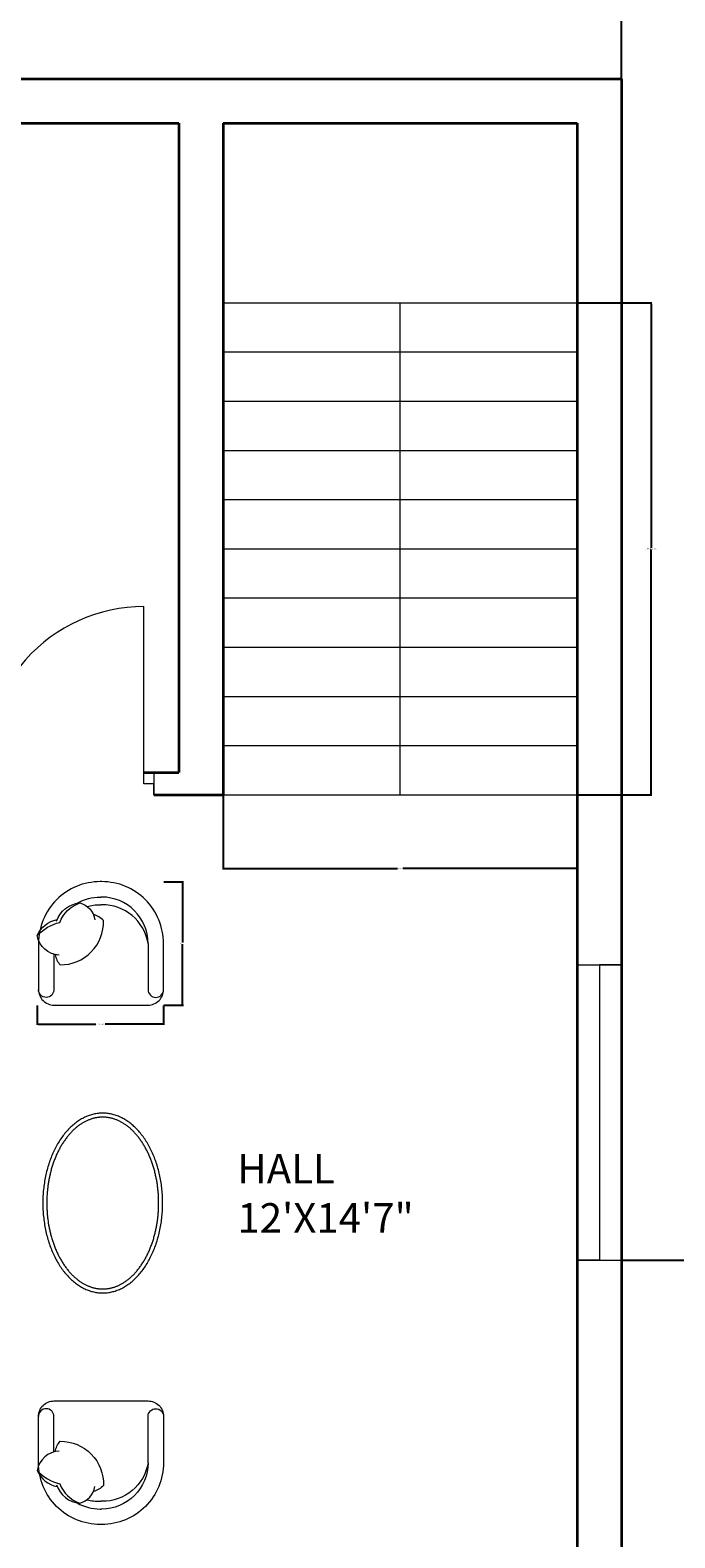
# Model space of a CAD drawing. Units: inches. Extents: x 2003 to 3241, y 1726 to 2849.
# Tile 3 of 7: x 2186 to 2317, y 2073 to 2380. Entities that reach past the tile are written whole.
import ezdxf

# ---------------------------------------------------------------- set-up
doc = ezdxf.new("R2010")
doc.units = ezdxf.units.IN
for name, color, linetype, lineweight in [('A-ANNO-DIMS', 2, 'Continuous', 18), ('A-AREA-IDEN', 7, 'Continuous', 18), ('A-DOOR', 3, 'Continuous', 18), ('A-FLOR-STRS', 7, 'Continuous', 18), ('A-FURN', 8, 'Continuous', 13), ('A-GLAZ', 4, 'Continuous', 18), ('A-WALL', 7, 'Continuous', 35)]:
    doc.layers.add(name, color=color, linetype=linetype, lineweight=lineweight)
doc.styles.get("Standard").update_dxf_attribs({"font": 'arial.ttf'})
doc.dimstyles.get("Standard").update_dxf_attribs({"dimtxt": 0.18, "dimasz": 0.18, "dimexe": 0.18, "dimexo": 0.0625, "dimgap": 0.09, "dimtad": 0, "dimtih": 1, "dimtoh": 1, "dimdec": 4, "dimzin": 0, "dimdsep": 46, "dimtxsty": 'Standard', "dimcen": 0.09, "dimadec": 0, "dimazin": 0, "dimtfac": 1, "dimtdec": 4, "dimtofl": 0, "dimtmove": 0, "dimatfit": 3, "dimfxl": 1, "dimtolj": 1, "dimtzin": 0, "dimarcsym": 0})

# ---------------------------------------------------------------- blocks, each defined once
blk = doc.blocks.new('WIN-60-HALL')
for p, q in [((0, 60), (9, 60)), ((9, 60), (4.5, 60)), ((4.5, 60), (4.5, 0)), ((4.5, 0), (0, 0)), ((0, 0), (9, 0)), ((9, 0), (9, 0))]:
    blk.add_line(p, q)
blk = doc.blocks.new('DOOR-BEDROOM')
for p, q in [((34.02, 2.25), (34.02, 38.25)), ((0, 4.5), (0, 0)), ((36.02, 4.5), (36.02, 0)), ((0, 0), (0, 2.25)), ((0, 2.25), (2, 2.25)), ((36.02, 2.25), (34.02, 2.25)), ((36.02, 0), (36.02, 2.25))]:
    blk.add_line(p, q)
blk.add_arc((34.02, 6.01), 32.24, 90, 186.689)
blk = doc.blocks.new('STAIR-GROUND-RUN')
for p, q in [((0, 100), (72, 100)), ((36, 97.06), (36, 100)), ((36, 0), (36, 97.06)), ((0, 90), (72, 90)), ((0, 80), (72, 80)), ((0, 70), (72, 70)), ((0, 60), (72, 60)), ((0, 50), (72, 50)), ((0, 40), (72, 40)), ((0, 30), (72, 30)), ((0, 20), (72, 20)), ((0, 10), (72, 10)), ((0, 0), (72, 0))]:
    blk.add_line(p, q)
blk = doc.blocks.new('CHAIR-LOUNGE')
at = {"ltscale": 0.03}
blk.add_lwpolyline([(12.96, 0), (22.53, 0, 0.414214), (25.67, 3.14), (25.67, 12.55, 0.414214), (13.12, 25.1), (12.96, 25.1), (12.81, 25.1, 0.414214), (0.26, 12.55), (0.26, 3.14, 0.414214), (3.39, 0), (12.96, 0)], format="xyb", dxfattribs=at)
for points in [[(8.13, 20.72, -0.130591), (12.81, 21.96), (12.96, 21.96)], [(22.53, 12.55, 0.414214), (13.12, 21.96), (12.96, 21.96)], [(0, 14.13, -0.14773), (4.58, 16.83, -0.213343), (8.63, 20.78, -0.178662)], [(3.7, 10.28, 0.165541), (4.67, 8.2, 0.425989), (13.48, 17.19, 0.121523), (11.39, 18.43, -7.115464)], [(3.95, 17.04, -0.306663), (8.63, 20.78, -0.30633), (11.69, 17.37, 0.872847)], [(10.13, 20.06, -0.072384), (12.81, 20.39), (12.96, 20.39)], [(22.53, 12.55, 0.372719), (13.12, 20.39), (12.96, 20.39)], [(4.49, 10.18, -0.356772), (0, 14.13, -0.249542), (4.07, 17.39, 9.61688)], [(22.53, 12.55), (22.53, 3.14, 0.414214), (24.1, 1.57), (24.1, 1.57, 0.414214), (25.67, 3.14)], [(3.39, 10.35), (3.39, 3.14, -0.414214), (1.83, 1.57), (1.83, 1.57, -0.414214), (0.26, 3.14)]]:
    blk.add_lwpolyline(points, format="xyb")
blk = doc.blocks.new('*D52')
at = {"layer": 'A-ANNO-DIMS', "color": 0, "lineweight": -2, "transparency": 16777216}
for p, q in [((2296.84, 2324.41), (2311.96, 2324.41)), ((2311.78, 2324.23), (2311.78, 2274.6)), ((2311.78, 2224.59), (2311.78, 2274.23)), ((2296.84, 2224.41), (2311.96, 2224.41))]:
    blk.add_line(p, q, dxfattribs=at)
at = {"layer": 'A-ANNO-DIMS', "color": 0, "transparency": 16777216}
for points in [[(2311.75, 2324.23), (2311.81, 2324.23), (2311.78, 2324.41)], [(2311.75, 2224.59), (2311.81, 2224.59), (2311.78, 2224.41)]]:
    blk.add_solid(points, dxfattribs=at)
at = {"layer": 'Defpoints', "color": 0, "transparency": 16777216}
for p in [(2296.78, 2324.41), (2311.78, 2324.41), (2296.78, 2224.41)]:
    blk.add_point(p, dxfattribs=at)
at = {"layer": 'A-ANNO-DIMS', "color": 0, "transparency": 16777216, "insert": (2311.78, 2274.41), "char_height": 0.18, "attachment_point": 5}
blk.add_mtext('\\A1;STAIR RUN 100 TYP.', dxfattribs=at)
blk = doc.blocks.new('*D53')
at = {"layer": 'A-ANNO-DIMS', "color": 0, "lineweight": -2, "transparency": 16777216}
for p, q in [((2224.78, 2224.35), (2224.78, 2209.23)), ((2296.78, 2224.35), (2296.78, 2209.23)), ((2224.96, 2209.41), (2260.25, 2209.41)), ((2296.6, 2209.41), (2261.31, 2209.41))]:
    blk.add_line(p, q, dxfattribs=at)
at = {"layer": 'A-ANNO-DIMS', "color": 0, "transparency": 16777216}
for points in [[(2224.96, 2209.44), (2224.96, 2209.38), (2224.78, 2209.41)], [(2296.6, 2209.44), (2296.6, 2209.38), (2296.78, 2209.41)]]:
    blk.add_solid(points, dxfattribs=at)
at = {"layer": 'Defpoints', "color": 0, "transparency": 16777216}
for p in [(2224.78, 2224.41), (2296.78, 2224.41), (2296.78, 2209.41)]:
    blk.add_point(p, dxfattribs=at)
at = {"layer": 'A-ANNO-DIMS', "color": 0, "transparency": 16777216, "insert": (2260.78, 2209.41), "char_height": 0.18, "attachment_point": 5}
blk.add_mtext('\\A1;72 TYP.', dxfattribs=at)
blk = doc.blocks.new('*D62')
at = {"layer": 'A-ANNO-DIMS', "color": 0, "lineweight": -2, "transparency": 16777216}
for p, q in [((2187.02, 2181.59), (2187.02, 2177.62)), ((2212.69, 2181.59), (2212.69, 2177.62)), ((2187.2, 2177.8), (2198.9, 2177.8)), ((2212.51, 2177.8), (2200.81, 2177.8))]:
    blk.add_line(p, q, dxfattribs=at)
at = {"layer": 'A-ANNO-DIMS', "color": 0, "transparency": 16777216}
for points in [[(2187.2, 2177.83), (2187.2, 2177.77), (2187.02, 2177.8)], [(2212.51, 2177.83), (2212.51, 2177.77), (2212.69, 2177.8)]]:
    blk.add_solid(points, dxfattribs=at)
at = {"layer": 'Defpoints', "color": 0, "transparency": 16777216}
for p in [(2187.02, 2181.65), (2212.69, 2181.65), (2212.69, 2177.8)]:
    blk.add_point(p, dxfattribs=at)
at = {"layer": 'A-ANNO-DIMS', "color": 0, "transparency": 16777216, "insert": (2199.85, 2177.8), "char_height": 0.18, "attachment_point": 5}
blk.add_mtext('\\A1;CHAIR 26 TYP.', dxfattribs=at)
blk = doc.blocks.new('*D63')
at = {"layer": 'A-ANNO-DIMS', "color": 0, "lineweight": -2, "transparency": 16777216}
for p, q in [((2212.75, 2206.75), (2216.72, 2206.75)), ((2216.54, 2206.57), (2216.54, 2194.38)), ((2216.54, 2181.83), (2216.54, 2194.02)), ((2212.75, 2181.65), (2216.72, 2181.65))]:
    blk.add_line(p, q, dxfattribs=at)
at = {"layer": 'A-ANNO-DIMS', "color": 0, "transparency": 16777216}
for points in [[(2216.51, 2206.57), (2216.57, 2206.57), (2216.54, 2206.75)], [(2216.51, 2181.83), (2216.57, 2181.83), (2216.54, 2181.65)]]:
    blk.add_solid(points, dxfattribs=at)
at = {"layer": 'Defpoints', "color": 0, "transparency": 16777216}
for p in [(2212.69, 2206.75), (2216.54, 2206.75), (2212.69, 2181.65)]:
    blk.add_point(p, dxfattribs=at)
at = {"layer": 'A-ANNO-DIMS', "color": 0, "transparency": 16777216, "insert": (2216.54, 2194.2), "char_height": 0.18, "attachment_point": 5}
blk.add_mtext('\\A1;25 TYP.', dxfattribs=at)
blk = doc.blocks.new('*D64')
at = {"layer": 'A-ANNO-DIMS', "color": 0, "lineweight": -2, "transparency": 16777216}
for p, q in [((2089.78, 2369.98), (2089.78, 2399.74)), ((2089.96, 2399.56), (2197.49, 2399.56)), ((2305.6, 2399.56), (2198.07, 2399.56)), ((2305.78, 2369.98), (2305.78, 2399.74))]:
    blk.add_line(p, q, dxfattribs=at)
at = {"layer": 'A-ANNO-DIMS', "color": 0, "transparency": 16777216}
for points in [[(2089.96, 2399.59), (2089.96, 2399.53), (2089.78, 2399.56)], [(2305.6, 2399.59), (2305.6, 2399.53), (2305.78, 2399.56)]]:
    blk.add_solid(points, dxfattribs=at)
at = {"layer": 'Defpoints', "color": 0, "transparency": 16777216}
for p in [(2305.78, 2399.56), (2089.78, 2369.91), (2305.78, 2369.91)]:
    blk.add_point(p, dxfattribs=at)
at = {"layer": 'A-ANNO-DIMS', "color": 0, "transparency": 16777216, "insert": (2197.78, 2399.56), "char_height": 0.18, "attachment_point": 5}
blk.add_mtext('\\A1;216', dxfattribs=at)
blk = doc.blocks.new('*D67')
at = {"layer": 'A-ANNO-DIMS', "color": 0, "lineweight": -2, "transparency": 16777216}
for p, q in [((2305.84, 2129.81), (2335.61, 2129.81)), ((2335.43, 2129.63), (2335.43, 2026.55)), ((2335.43, 1923.09), (2335.43, 2026.18)), ((2305.84, 1922.91), (2335.61, 1922.91))]:
    blk.add_line(p, q, dxfattribs=at)
at = {"layer": 'A-ANNO-DIMS', "color": 0, "transparency": 16777216}
for points in [[(2335.4, 2129.63), (2335.46, 2129.63), (2335.43, 2129.81)], [(2335.4, 1923.09), (2335.46, 1923.09), (2335.43, 1922.91)]]:
    blk.add_solid(points, dxfattribs=at)
at = {"layer": 'Defpoints', "color": 0, "transparency": 16777216}
for p in [(2305.78, 2129.81), (2335.43, 2129.81), (2305.78, 1922.91)]:
    blk.add_point(p, dxfattribs=at)
at = {"layer": 'A-ANNO-DIMS', "color": 0, "transparency": 16777216, "insert": (2335.43, 2026.36), "char_height": 0.18, "attachment_point": 5}
blk.add_mtext('\\A1;206.9', dxfattribs=at)

msp = doc.modelspace()

# ---------------------------------------------------------------- linework, layer by layer
at = {"layer": 'A-FURN', "ltscale": 0.03}
msp.add_polyline3d([(2200.3301, 2159.6931, 0), (2200.0996, 2159.6898, 0), (2199.8692, 2159.68, 0), (2199.639, 2159.6637, 0), (2199.409, 2159.6408, 0), (2199.1794, 2159.6114, 0), (2198.9501, 2159.5755, 0), (2198.7214, 2159.533, 0), (2198.4932, 2159.4841, 0), (2198.2657, 2159.4287, 0), (2198.0389, 2159.3669, 0), (2197.813, 2159.2987, 0), (2197.5879, 2159.224, 0), (2197.3638, 2159.143, 0), (2197.1408, 2159.0556, 0), (2196.919, 2158.9619, 0), (2196.6983, 2158.862, 0), (2196.479, 2158.7557, 0), (2196.261, 2158.6433, 0), (2196.0445, 2158.5247, 0), (2195.8296, 2158.4, 0), (2195.6162, 2158.2692, 0), (2195.4045, 2158.1324, 0), (2195.1946, 2157.9896, 0), (2194.9866, 2157.8409, 0), (2194.7804, 2157.6862, 0), (2194.5762, 2157.5258, 0), (2194.3741, 2157.3596, 0), (2194.1742, 2157.1876, 0), (2193.9764, 2157.0101, 0), (2193.7809, 2156.8269, 0), (2193.5878, 2156.6383, 0), (2193.397, 2156.4442, 0), (2193.2088, 2156.2447, 0), (2193.0231, 2156.0399, 0), (2192.84, 2155.8298, 0), (2192.6596, 2155.6146, 0), (2192.482, 2155.3944, 0), (2192.3071, 2155.1691, 0), (2192.1352, 2154.9389, 0), (2191.9661, 2154.7038, 0), (2191.8001, 2154.464, 0), (2191.6371, 2154.2196, 0), (2191.4773, 2153.9705, 0), (2191.3206, 2153.717, 0), (2191.1671, 2153.459, 0), (2191.0169, 2153.1968, 0), (2190.87, 2152.9303, 0), (2190.7266, 2152.6597, 0), (2190.5866, 2152.3851, 0), (2190.45, 2152.1065, 0), (2190.317, 2151.8242, 0), (2190.1876, 2151.5381, 0), (2190.0618, 2151.2483, 0), (2189.9397, 2150.9551, 0), (2189.8214, 2150.6585, 0), (2189.7068, 2150.3585, 0), (2189.5959, 2150.0553, 0), (2189.489, 2149.7491, 0), (2189.3859, 2149.4399, 0), (2189.2867, 2149.1278, 0), (2189.1915, 2148.8129, 0), (2189.1003, 2148.4954, 0), (2189.0131, 2148.1754, 0), (2188.93, 2147.8529, 0), (2188.8509, 2147.5282, 0), (2188.776, 2147.2012, 0), (2188.7052, 2146.8722, 0), (2188.6385, 2146.5412, 0), (2188.5761, 2146.2084, 0), (2188.5178, 2145.8739, 0), (2188.4638, 2145.5378, 0), (2188.414, 2145.2002, 0), (2188.3685, 2144.8613, 0), (2188.3273, 2144.5212, 0), (2188.2904, 2144.1799, 0), (2188.2578, 2143.8376, 0), (2188.2295, 2143.4945, 0), (2188.2055, 2143.1507, 0), (2188.1859, 2142.8062, 0), (2188.1707, 2142.4612, 0), (2188.1598, 2142.1159, 0), (2188.1532, 2141.7703, 0), (2188.1511, 2141.4246, 0), (2188.1532, 2141.0788, 0), (2188.1598, 2140.7332, 0), (2188.1707, 2140.3879, 0), (2188.1859, 2140.0429, 0), (2188.2055, 2139.6984, 0), (2188.2295, 2139.3546, 0), (2188.2578, 2139.0115, 0), (2188.2904, 2138.6692, 0), (2188.3273, 2138.3279, 0), (2188.3685, 2137.9878, 0), (2188.414, 2137.6489, 0), (2188.4638, 2137.3113, 0), (2188.5178, 2136.9752, 0), (2188.5761, 2136.6407, 0), (2188.6385, 2136.3079, 0), (2188.7052, 2135.9769, 0), (2188.776, 2135.6479, 0), (2188.8509, 2135.3209, 0), (2188.93, 2134.9962, 0), (2189.0131, 2134.6737, 0), (2189.1003, 2134.3537, 0), (2189.1915, 2134.0362, 0), (2189.2867, 2133.7213, 0), (2189.3859, 2133.4092, 0), (2189.489, 2133.1, 0), (2189.5959, 2132.7938, 0), (2189.7068, 2132.4906, 0), (2189.8214, 2132.1906, 0), (2189.9397, 2131.894, 0), (2190.0618, 2131.6008, 0), (2190.1876, 2131.311, 0), (2190.317, 2131.025, 0), (2190.45, 2130.7426, 0), (2190.5866, 2130.464, 0), (2190.7266, 2130.1894, 0), (2190.87, 2129.9188, 0), (2191.0169, 2129.6523, 0), (2191.1671, 2129.3901, 0), (2191.3206, 2129.1321, 0), (2191.4773, 2128.8786, 0), (2191.6371, 2128.6295, 0), (2191.8001, 2128.3851, 0), (2191.9661, 2128.1453, 0), (2192.1352, 2127.9102, 0), (2192.3071, 2127.68, 0), (2192.482, 2127.4547, 0), (2192.6596, 2127.2345, 0), (2192.84, 2127.0193, 0), (2193.0231, 2126.8092, 0), (2193.2088, 2126.6044, 0), (2193.397, 2126.4049, 0), (2193.5878, 2126.2108, 0), (2193.7809, 2126.0222, 0), (2193.9764, 2125.839, 0), (2194.1742, 2125.6615, 0), (2194.3741, 2125.4895, 0), (2194.5762, 2125.3233, 0), (2194.7804, 2125.1629, 0), (2194.9866, 2125.0082, 0), (2195.1946, 2124.8595, 0), (2195.4045, 2124.7167, 0), (2195.6162, 2124.5799, 0), (2195.8296, 2124.4491, 0), (2196.0445, 2124.3244, 0), (2196.261, 2124.2058, 0), (2196.479, 2124.0934, 0), (2196.6983, 2123.9871, 0), (2196.919, 2123.8872, 0), (2197.1408, 2123.7935, 0), (2197.3638, 2123.7061, 0), (2197.5879, 2123.6251, 0), (2197.813, 2123.5504, 0), (2198.0389, 2123.4822, 0), (2198.2657, 2123.4204, 0), (2198.4932, 2123.365, 0), (2198.7214, 2123.3161, 0), (2198.9501, 2123.2736, 0), (2199.1794, 2123.2377, 0), (2199.409, 2123.2083, 0), (2199.639, 2123.1854, 0), (2199.8692, 2123.1691, 0), (2200.0996, 2123.1593, 0), (2200.3301, 2123.156, 0), (2200.5606, 2123.1593, 0), (2200.791, 2123.1691, 0), (2201.0212, 2123.1854, 0), (2201.2512, 2123.2083, 0), (2201.4808, 2123.2377, 0), (2201.7101, 2123.2736, 0), (2201.9388, 2123.3161, 0), (2202.167, 2123.365, 0), (2202.3945, 2123.4204, 0), (2202.6213, 2123.4822, 0), (2202.8472, 2123.5504, 0), (2203.0723, 2123.6251, 0), (2203.2964, 2123.7061, 0), (2203.5194, 2123.7935, 0), (2203.7412, 2123.8872, 0), (2203.9619, 2123.9871, 0), (2204.1812, 2124.0934, 0), (2204.3992, 2124.2058, 0), (2204.6157, 2124.3244, 0), (2204.8306, 2124.4491, 0), (2205.044, 2124.5799, 0), (2205.2557, 2124.7167, 0), (2205.4656, 2124.8595, 0), (2205.6736, 2125.0082, 0), (2205.8798, 2125.1629, 0), (2206.084, 2125.3233, 0), (2206.2861, 2125.4895, 0), (2206.486, 2125.6615, 0), (2206.6838, 2125.839, 0), (2206.8793, 2126.0222, 0), (2207.0724, 2126.2108, 0), (2207.2632, 2126.4049, 0), (2207.4514, 2126.6044, 0), (2207.6371, 2126.8092, 0), (2207.8202, 2127.0193, 0), (2208.0006, 2127.2345, 0), (2208.1782, 2127.4547, 0), (2208.3531, 2127.68, 0), (2208.525, 2127.9102, 0), (2208.6941, 2128.1453, 0), (2208.8601, 2128.3851, 0), (2209.0231, 2128.6295, 0), (2209.183, 2128.8786, 0), (2209.3396, 2129.1321, 0), (2209.4931, 2129.3901, 0), (2209.6433, 2129.6523, 0), (2209.7902, 2129.9188, 0), (2209.9336, 2130.1894, 0), (2210.0736, 2130.464, 0), (2210.2102, 2130.7426, 0), (2210.3432, 2131.025, 0), (2210.4726, 2131.311, 0), (2210.5984, 2131.6008, 0), (2210.7205, 2131.894, 0), (2210.8388, 2132.1906, 0), (2210.9534, 2132.4906, 0), (2211.0643, 2132.7938, 0), (2211.1712, 2133.1, 0), (2211.2743, 2133.4092, 0), (2211.3735, 2133.7213, 0), (2211.4687, 2134.0362, 0), (2211.5599, 2134.3537, 0), (2211.6471, 2134.6737, 0), (2211.7302, 2134.9962, 0), (2211.8093, 2135.3209, 0), (2211.8842, 2135.6479, 0), (2211.955, 2135.9769, 0), (2212.0217, 2136.3079, 0), (2212.0841, 2136.6407, 0), (2212.1424, 2136.9752, 0), (2212.1964, 2137.3113, 0), (2212.2462, 2137.6489, 0), (2212.2917, 2137.9878, 0), (2212.3329, 2138.3279, 0), (2212.3698, 2138.6692, 0), (2212.4024, 2139.0115, 0), (2212.4307, 2139.3546, 0), (2212.4547, 2139.6984, 0), (2212.4743, 2140.0429, 0), (2212.4895, 2140.3879, 0), (2212.5004, 2140.7332, 0), (2212.507, 2141.0788, 0), (2212.5091, 2141.4246, 0), (2212.507, 2141.7703, 0), (2212.5004, 2142.1159, 0), (2212.4895, 2142.4612, 0), (2212.4743, 2142.8062, 0), (2212.4547, 2143.1507, 0), (2212.4307, 2143.4945, 0), (2212.4024, 2143.8376, 0), (2212.3698, 2144.1799, 0), (2212.3329, 2144.5212, 0), (2212.2917, 2144.8613, 0), (2212.2462, 2145.2002, 0), (2212.1964, 2145.5378, 0), (2212.1424, 2145.8739, 0), (2212.0841, 2146.2084, 0), (2212.0217, 2146.5412, 0), (2211.955, 2146.8722, 0), (2211.8842, 2147.2012, 0), (2211.8093, 2147.5282, 0), (2211.7302, 2147.8529, 0), (2211.6471, 2148.1754, 0), (2211.5599, 2148.4954, 0), (2211.4687, 2148.8129, 0), (2211.3735, 2149.1278, 0), (2211.2743, 2149.4399, 0), (2211.1712, 2149.7491, 0), (2211.0643, 2150.0553, 0), (2210.9534, 2150.3585, 0), (2210.8388, 2150.6585, 0), (2210.7205, 2150.9551, 0), (2210.5984, 2151.2483, 0), (2210.4726, 2151.5381, 0), (2210.3432, 2151.8242, 0), (2210.2102, 2152.1065, 0), (2210.0736, 2152.3851, 0), (2209.9336, 2152.6597, 0), (2209.7902, 2152.9303, 0), (2209.6433, 2153.1968, 0), (2209.4931, 2153.459, 0), (2209.3396, 2153.717, 0), (2209.183, 2153.9705, 0), (2209.0231, 2154.2196, 0), (2208.8601, 2154.464, 0), (2208.6941, 2154.7038, 0), (2208.525, 2154.9389, 0), (2208.3531, 2155.1691, 0), (2208.1782, 2155.3944, 0), (2208.0006, 2155.6146, 0), (2207.8202, 2155.8298, 0), (2207.6371, 2156.0399, 0), (2207.4514, 2156.2447, 0), (2207.2632, 2156.4442, 0), (2207.0724, 2156.6383, 0), (2206.8793, 2156.8269, 0), (2206.6838, 2157.0101, 0), (2206.486, 2157.1876, 0), (2206.2861, 2157.3596, 0), (2206.084, 2157.5258, 0), (2205.8798, 2157.6862, 0), (2205.6736, 2157.8409, 0), (2205.4656, 2157.9896, 0), (2205.2557, 2158.1324, 0), (2205.044, 2158.2692, 0), (2204.8306, 2158.4, 0), (2204.6157, 2158.5247, 0), (2204.3992, 2158.6433, 0), (2204.1812, 2158.7557, 0), (2203.9619, 2158.862, 0), (2203.7412, 2158.9619, 0), (2203.5194, 2159.0556, 0), (2203.2964, 2159.143, 0), (2203.0723, 2159.224, 0), (2202.8472, 2159.2987, 0), (2202.6213, 2159.3669, 0), (2202.3945, 2159.4287, 0), (2202.167, 2159.4841, 0), (2201.9388, 2159.533, 0), (2201.7101, 2159.5755, 0), (2201.4808, 2159.6114, 0), (2201.2512, 2159.6408, 0), (2201.0212, 2159.6637, 0), (2200.791, 2159.68, 0), (2200.5606, 2159.6898, 0), (2200.3301, 2159.6931, 0)], dxfattribs=at)
at = {"layer": 'A-FURN'}
msp.add_polyline3d([(2200.3301, 2158.8812, 0), (2200.2055, 2158.8801, 0), (2200.0804, 2158.8769, 0), (2199.9547, 2158.8715, 0), (2199.8285, 2158.8639, 0), (2199.7018, 2158.8541, 0), (2199.5745, 2158.842, 0), (2199.4468, 2158.8277, 0), (2199.3185, 2158.811, 0), (2199.1899, 2158.792, 0), (2199.0608, 2158.7706, 0), (2198.9312, 2158.7468, 0), (2198.8013, 2158.7205, 0), (2198.671, 2158.6919, 0), (2198.5403, 2158.6607, 0), (2198.4093, 2158.627, 0), (2198.278, 2158.5908, 0), (2198.1463, 2158.552, 0), (2198.0143, 2158.5106, 0), (2197.8821, 2158.4666, 0), (2197.7496, 2158.4199, 0), (2197.6169, 2158.3706, 0), (2197.4839, 2158.3185, 0), (2197.3508, 2158.2637, 0), (2197.2175, 2158.2061, 0), (2197.0842, 2158.1457, 0), (2196.9508, 2158.0826, 0), (2196.8175, 2158.0167, 0), (2196.6841, 2157.948, 0), (2196.5509, 2157.8765, 0), (2196.4177, 2157.8023, 0), (2196.2847, 2157.7252, 0), (2196.1519, 2157.6454, 0), (2196.0193, 2157.5628, 0), (2195.887, 2157.4774, 0), (2195.755, 2157.3892, 0), (2195.6234, 2157.2981, 0), (2195.4921, 2157.2043, 0), (2195.3613, 2157.1076, 0), (2195.2309, 2157.0082, 0), (2195.1011, 2156.9059, 0), (2194.9718, 2156.8007, 0), (2194.8431, 2156.6927, 0), (2194.715, 2156.5817, 0), (2194.5876, 2156.4677, 0), (2194.4608, 2156.3506, 0), (2194.3348, 2156.2307, 0), (2194.2095, 2156.1078, 0), (2194.085, 2155.982, 0), (2193.9613, 2155.8535, 0), (2193.8385, 2155.7221, 0), (2193.7165, 2155.588, 0), (2193.5955, 2155.4513, 0), (2193.4754, 2155.3118, 0), (2193.3563, 2155.1698, 0), (2193.2382, 2155.0252, 0), (2193.1212, 2154.8781, 0), (2193.0052, 2154.7285, 0), (2192.8904, 2154.5765, 0), (2192.7767, 2154.422, 0), (2192.6642, 2154.2652, 0), (2192.5529, 2154.1062, 0), (2192.4429, 2153.9448, 0), (2192.3341, 2153.7812, 0), (2192.2267, 2153.6154, 0), (2192.1206, 2153.4475, 0), (2192.0159, 2153.2775, 0), (2191.9126, 2153.1055, 0), (2191.8108, 2152.9314, 0), (2191.7104, 2152.7554, 0), (2191.6116, 2152.5774, 0), (2191.5143, 2152.3975, 0), (2191.4186, 2152.2158, 0), (2191.3245, 2152.0323, 0), (2191.2321, 2151.8471, 0), (2191.1413, 2151.6601, 0), (2191.0523, 2151.4715, 0), (2190.965, 2151.2812, 0), (2190.8795, 2151.0893, 0), (2190.7958, 2150.8959, 0), (2190.7139, 2150.701, 0), (2190.634, 2150.5046, 0), (2190.5559, 2150.3069, 0), (2190.4798, 2150.1077, 0), (2190.4057, 2149.9075, 0), (2190.3336, 2149.7066, 0), (2190.2634, 2149.5053, 0), (2190.1951, 2149.3034, 0), (2190.1288, 2149.101, 0), (2190.0644, 2148.8981, 0), (2190.002, 2148.6946, 0), (2189.9415, 2148.4907, 0), (2189.8828, 2148.2864, 0), (2189.8261, 2148.0816, 0), (2189.7713, 2147.8763, 0), (2189.7183, 2147.6706, 0), (2189.6672, 2147.4646, 0), (2189.618, 2147.2581, 0), (2189.5707, 2147.0512, 0), (2189.5251, 2146.844, 0), (2189.4815, 2146.6364, 0), (2189.4396, 2146.4285, 0), (2189.3996, 2146.2202, 0), (2189.3614, 2146.0116, 0), (2189.325, 2145.8028, 0), (2189.2904, 2145.5936, 0), (2189.2576, 2145.3842, 0), (2189.2266, 2145.1745, 0), (2189.1973, 2144.9645, 0), (2189.1698, 2144.7544, 0), (2189.1441, 2144.544, 0), (2189.1201, 2144.3334, 0), (2189.0979, 2144.1226, 0), (2189.0773, 2143.9117, 0), (2189.0585, 2143.7006, 0), (2189.0415, 2143.4893, 0), (2189.0261, 2143.2779, 0), (2189.0124, 2143.0664, 0), (2189.0004, 2142.8548, 0), (2188.9901, 2142.643, 0), (2188.9815, 2142.4312, 0), (2188.9745, 2142.2194, 0), (2188.9692, 2142.0075, 0), (2188.9655, 2141.7955, 0), (2188.9635, 2141.5835, 0), (2188.963, 2141.3716, 0), (2188.9643, 2141.1596, 0), (2188.9671, 2140.9476, 0), (2188.9716, 2140.7357, 0), (2188.9778, 2140.5238, 0), (2188.9856, 2140.3119, 0), (2188.995, 2140.1002, 0), (2189.0062, 2139.8885, 0), (2189.019, 2139.6769, 0), (2189.0336, 2139.4655, 0), (2189.0498, 2139.2541, 0), (2189.0677, 2139.043, 0), (2189.0874, 2138.8319, 0), (2189.1088, 2138.6211, 0), (2189.1319, 2138.4104, 0), (2189.1567, 2138.1999, 0), (2189.1834, 2137.9896, 0), (2189.2117, 2137.7796, 0), (2189.2419, 2137.5697, 0), (2189.2738, 2137.3602, 0), (2189.3075, 2137.1509, 0), (2189.343, 2136.9419, 0), (2189.3803, 2136.7331, 0), (2189.4194, 2136.5247, 0), (2189.4603, 2136.3166, 0), (2189.5031, 2136.1089, 0), (2189.5477, 2135.9015, 0), (2189.5941, 2135.6944, 0), (2189.6424, 2135.4877, 0), (2189.6925, 2135.2814, 0), (2189.7446, 2135.0756, 0), (2189.7985, 2134.8701, 0), (2189.8542, 2134.6651, 0), (2189.9119, 2134.4605, 0), (2189.9715, 2134.2564, 0), (2190.033, 2134.0527, 0), (2190.0964, 2133.8495, 0), (2190.1617, 2133.6469, 0), (2190.229, 2133.4447, 0), (2190.2982, 2133.2431, 0), (2190.3694, 2133.042, 0), (2190.4425, 2132.8415, 0), (2190.5176, 2132.6417, 0), (2190.5947, 2132.4432, 0), (2190.6737, 2132.2461, 0), (2190.7546, 2132.0504, 0), (2190.8374, 2131.8563, 0), (2190.922, 2131.6636, 0), (2191.0084, 2131.4726, 0), (2191.0966, 2131.2831, 0), (2191.1865, 2131.0953, 0), (2191.2781, 2130.9092, 0), (2191.3713, 2130.7248, 0), (2191.4662, 2130.5422, 0), (2191.5627, 2130.3614, 0), (2191.6608, 2130.1825, 0), (2191.7604, 2130.0055, 0), (2191.8615, 2129.8304, 0), (2191.9641, 2129.6573, 0), (2192.0681, 2129.4863, 0), (2192.1735, 2129.3173, 0), (2192.2802, 2129.1505, 0), (2192.3883, 2128.9858, 0), (2192.4977, 2128.8233, 0), (2192.6084, 2128.6631, 0), (2192.7203, 2128.5052, 0), (2192.8334, 2128.3496, 0), (2192.9476, 2128.1963, 0), (2193.063, 2128.0455, 0), (2193.1795, 2127.8971, 0), (2193.2971, 2127.7513, 0), (2193.4157, 2127.608, 0), (2193.5353, 2127.4672, 0), (2193.6559, 2127.3291, 0), (2193.7774, 2127.1937, 0), (2193.8998, 2127.061, 0), (2194.023, 2126.931, 0), (2194.1471, 2126.8038, 0), (2194.272, 2126.6795, 0), (2194.3977, 2126.5581, 0), (2194.5241, 2126.4396, 0), (2194.6512, 2126.324, 0), (2194.779, 2126.2115, 0), (2194.9074, 2126.102, 0), (2195.0364, 2125.9955, 0), (2195.1659, 2125.8917, 0), (2195.296, 2125.7909, 0), (2195.4266, 2125.6928, 0), (2195.5577, 2125.5975, 0), (2195.6891, 2125.5051, 0), (2195.821, 2125.4155, 0), (2195.9531, 2125.3287, 0), (2196.0856, 2125.2446, 0), (2196.2183, 2125.1634, 0), (2196.3512, 2125.085, 0), (2196.4843, 2125.0094, 0), (2196.6175, 2124.9365, 0), (2196.7508, 2124.8664, 0), (2196.8842, 2124.7991, 0), (2197.0175, 2124.7346, 0), (2197.1509, 2124.6729, 0), (2197.2842, 2124.6139, 0), (2197.4174, 2124.5577, 0), (2197.5504, 2124.5042, 0), (2197.6833, 2124.4535, 0), (2197.8159, 2124.4055, 0), (2197.9483, 2124.3602, 0), (2198.0804, 2124.3175, 0), (2198.2122, 2124.2774, 0), (2198.3437, 2124.2399, 0), (2198.4749, 2124.2049, 0), (2198.6057, 2124.1725, 0), (2198.7362, 2124.1426, 0), (2198.8663, 2124.1151, 0), (2198.9961, 2124.0901, 0), (2199.1254, 2124.0675, 0), (2199.2543, 2124.0473, 0), (2199.3827, 2124.0295, 0), (2199.5107, 2124.014, 0), (2199.6382, 2124.0007, 0), (2199.7652, 2123.9898, 0), (2199.8917, 2123.9811, 0), (2200.0176, 2123.9746, 0), (2200.1431, 2123.9703, 0), (2200.2679, 2123.9682, 0), (2200.3923, 2123.9682, 0), (2200.5171, 2123.9703, 0), (2200.6426, 2123.9746, 0), (2200.7685, 2123.9811, 0), (2200.895, 2123.9898, 0), (2201.022, 2124.0007, 0), (2201.1495, 2124.014, 0), (2201.2775, 2124.0295, 0), (2201.4059, 2124.0473, 0), (2201.5348, 2124.0675, 0), (2201.6641, 2124.0901, 0), (2201.7939, 2124.1151, 0), (2201.924, 2124.1426, 0), (2202.0545, 2124.1725, 0), (2202.1853, 2124.2049, 0), (2202.3165, 2124.2399, 0), (2202.448, 2124.2774, 0), (2202.5798, 2124.3175, 0), (2202.7119, 2124.3602, 0), (2202.8443, 2124.4055, 0), (2202.9769, 2124.4535, 0), (2203.1098, 2124.5042, 0), (2203.2428, 2124.5577, 0), (2203.376, 2124.6139, 0), (2203.5093, 2124.6729, 0), (2203.6427, 2124.7346, 0), (2203.776, 2124.7991, 0), (2203.9094, 2124.8664, 0), (2204.0427, 2124.9365, 0), (2204.1759, 2125.0094, 0), (2204.309, 2125.085, 0), (2204.4419, 2125.1634, 0), (2204.5746, 2125.2446, 0), (2204.7071, 2125.3287, 0), (2204.8392, 2125.4155, 0), (2204.9711, 2125.5051, 0), (2205.1025, 2125.5975, 0), (2205.2336, 2125.6928, 0), (2205.3642, 2125.7909, 0), (2205.4943, 2125.8917, 0), (2205.6238, 2125.9955, 0), (2205.7528, 2126.102, 0), (2205.8812, 2126.2115, 0), (2206.009, 2126.324, 0), (2206.1361, 2126.4396, 0), (2206.2625, 2126.5581, 0), (2206.3882, 2126.6795, 0), (2206.5131, 2126.8038, 0), (2206.6372, 2126.931, 0), (2206.7604, 2127.061, 0), (2206.8828, 2127.1937, 0), (2207.0043, 2127.3291, 0), (2207.1249, 2127.4672, 0), (2207.2445, 2127.608, 0), (2207.3631, 2127.7513, 0), (2207.4807, 2127.8971, 0), (2207.5972, 2128.0455, 0), (2207.7126, 2128.1963, 0), (2207.8268, 2128.3496, 0), (2207.9399, 2128.5052, 0), (2208.0518, 2128.6631, 0), (2208.1625, 2128.8233, 0), (2208.2719, 2128.9858, 0), (2208.38, 2129.1505, 0), (2208.4867, 2129.3173, 0), (2208.5921, 2129.4863, 0), (2208.6961, 2129.6573, 0), (2208.7987, 2129.8304, 0), (2208.8998, 2130.0055, 0), (2208.9994, 2130.1825, 0), (2209.0975, 2130.3614, 0), (2209.194, 2130.5422, 0), (2209.2889, 2130.7248, 0), (2209.3821, 2130.9092, 0), (2209.4737, 2131.0953, 0), (2209.5636, 2131.2831, 0), (2209.6518, 2131.4726, 0), (2209.7382, 2131.6636, 0), (2209.8228, 2131.8563, 0), (2209.9056, 2132.0504, 0), (2209.9865, 2132.2461, 0), (2210.0655, 2132.4432, 0), (2210.1426, 2132.6417, 0), (2210.2177, 2132.8415, 0), (2210.2908, 2133.042, 0), (2210.362, 2133.2431, 0), (2210.4312, 2133.4447, 0), (2210.4985, 2133.6469, 0), (2210.5638, 2133.8495, 0), (2210.6272, 2134.0527, 0), (2210.6887, 2134.2564, 0), (2210.7483, 2134.4605, 0), (2210.806, 2134.6651, 0), (2210.8617, 2134.8701, 0), (2210.9156, 2135.0756, 0), (2210.9677, 2135.2814, 0), (2211.0178, 2135.4877, 0), (2211.0661, 2135.6944, 0), (2211.1125, 2135.9015, 0), (2211.1571, 2136.1089, 0), (2211.1999, 2136.3166, 0), (2211.2408, 2136.5247, 0), (2211.2799, 2136.7331, 0), (2211.3172, 2136.9419, 0), (2211.3527, 2137.1509, 0), (2211.3864, 2137.3602, 0), (2211.4183, 2137.5697, 0), (2211.4485, 2137.7796, 0), (2211.4768, 2137.9896, 0), (2211.5035, 2138.1999, 0), (2211.5283, 2138.4104, 0), (2211.5514, 2138.6211, 0), (2211.5728, 2138.8319, 0), (2211.5925, 2139.043, 0), (2211.6104, 2139.2541, 0), (2211.6266, 2139.4655, 0), (2211.6412, 2139.6769, 0), (2211.654, 2139.8885, 0), (2211.6652, 2140.1002, 0), (2211.6746, 2140.3119, 0), (2211.6824, 2140.5238, 0), (2211.6886, 2140.7357, 0), (2211.6931, 2140.9476, 0), (2211.6959, 2141.1596, 0), (2211.6972, 2141.3716, 0), (2211.6967, 2141.5835, 0), (2211.6947, 2141.7955, 0), (2211.691, 2142.0075, 0), (2211.6857, 2142.2194, 0), (2211.6787, 2142.4312, 0), (2211.6701, 2142.643, 0), (2211.6598, 2142.8548, 0), (2211.6478, 2143.0664, 0), (2211.6341, 2143.2779, 0), (2211.6187, 2143.4893, 0), (2211.6017, 2143.7006, 0), (2211.5829, 2143.9117, 0), (2211.5623, 2144.1226, 0), (2211.5401, 2144.3334, 0), (2211.5161, 2144.544, 0), (2211.4904, 2144.7544, 0), (2211.4629, 2144.9645, 0), (2211.4336, 2145.1745, 0), (2211.4026, 2145.3842, 0), (2211.3698, 2145.5936, 0), (2211.3352, 2145.8028, 0), (2211.2988, 2146.0116, 0), (2211.2606, 2146.2202, 0), (2211.2206, 2146.4285, 0), (2211.1787, 2146.6364, 0), (2211.1351, 2146.844, 0), (2211.0895, 2147.0512, 0), (2211.0422, 2147.2581, 0), (2210.993, 2147.4646, 0), (2210.9419, 2147.6706, 0), (2210.8889, 2147.8763, 0), (2210.8341, 2148.0816, 0), (2210.7774, 2148.2864, 0), (2210.7187, 2148.4907, 0), (2210.6582, 2148.6946, 0), (2210.5958, 2148.8981, 0), (2210.5314, 2149.101, 0), (2210.4651, 2149.3034, 0), (2210.3968, 2149.5053, 0), (2210.3266, 2149.7066, 0), (2210.2545, 2149.9075, 0), (2210.1804, 2150.1077, 0), (2210.1043, 2150.3069, 0), (2210.0262, 2150.5046, 0), (2209.9463, 2150.701, 0), (2209.8644, 2150.8959, 0), (2209.7807, 2151.0893, 0), (2209.6952, 2151.2812, 0), (2209.6079, 2151.4715, 0), (2209.5189, 2151.6601, 0), (2209.4281, 2151.8471, 0), (2209.3357, 2152.0323, 0), (2209.2416, 2152.2158, 0), (2209.1459, 2152.3975, 0), (2209.0486, 2152.5774, 0), (2208.9498, 2152.7554, 0), (2208.8494, 2152.9314, 0), (2208.7476, 2153.1055, 0), (2208.6443, 2153.2775, 0), (2208.5396, 2153.4475, 0), (2208.4335, 2153.6154, 0), (2208.3261, 2153.7812, 0), (2208.2173, 2153.9448, 0), (2208.1073, 2154.1062, 0), (2207.996, 2154.2652, 0), (2207.8835, 2154.422, 0), (2207.7698, 2154.5765, 0), (2207.655, 2154.7285, 0), (2207.539, 2154.8781, 0), (2207.422, 2155.0252, 0), (2207.3039, 2155.1698, 0), (2207.1848, 2155.3118, 0), (2207.0647, 2155.4513, 0), (2206.9437, 2155.588, 0), (2206.8217, 2155.7221, 0), (2206.6989, 2155.8535, 0), (2206.5752, 2155.982, 0), (2206.4507, 2156.1078, 0), (2206.3254, 2156.2307, 0), (2206.1994, 2156.3506, 0), (2206.0726, 2156.4677, 0), (2205.9452, 2156.5817, 0), (2205.8171, 2156.6927, 0), (2205.6884, 2156.8007, 0), (2205.5591, 2156.9059, 0), (2205.4293, 2157.0082, 0), (2205.2989, 2157.1076, 0), (2205.1681, 2157.2043, 0), (2205.0368, 2157.2981, 0), (2204.9052, 2157.3892, 0), (2204.7732, 2157.4774, 0), (2204.6409, 2157.5628, 0), (2204.5083, 2157.6454, 0), (2204.3755, 2157.7252, 0), (2204.2425, 2157.8023, 0), (2204.1093, 2157.8765, 0), (2203.9761, 2157.948, 0), (2203.8427, 2158.0167, 0), (2203.7094, 2158.0826, 0), (2203.576, 2158.1457, 0), (2203.4427, 2158.2061, 0), (2203.3094, 2158.2637, 0), (2203.1763, 2158.3185, 0), (2203.0433, 2158.3706, 0), (2202.9106, 2158.4199, 0), (2202.7781, 2158.4666, 0), (2202.6459, 2158.5106, 0), (2202.5139, 2158.552, 0), (2202.3822, 2158.5908, 0), (2202.2509, 2158.627, 0), (2202.1199, 2158.6607, 0), (2201.9892, 2158.6919, 0), (2201.8589, 2158.7205, 0), (2201.729, 2158.7468, 0), (2201.5994, 2158.7706, 0), (2201.4703, 2158.792, 0), (2201.3417, 2158.811, 0), (2201.2134, 2158.8277, 0), (2201.0857, 2158.842, 0), (2200.9584, 2158.8541, 0), (2200.8317, 2158.8639, 0), (2200.7055, 2158.8715, 0), (2200.5798, 2158.8769, 0), (2200.4547, 2158.8801, 0), (2200.3301, 2158.8812, 0)], dxfattribs=at)
at = {"layer": 'A-WALL'}
for p, q in [((2089.7784, 2369.9135), (2305.7784, 2369.9135)), ((2089.7784, 2369.9135), (2305.7784, 2369.9135)), ((2305.7784, 2369.9135), (2305.7784, 1922.9135)), ((2098.7784, 2360.9135), (2215.7784, 2360.9135)), ((2215.7784, 2360.9135), (2215.7784, 2228.9135)), ((2224.7784, 2360.9135), (2224.7784, 2228.9135)), ((2224.7784, 2360.9135), (2296.7784, 2360.9135)), ((2296.7784, 2360.9135), (2296.7784, 2228.9135)), ((2208.723, 2228.9135), (2215.7784, 2228.9135)), ((2224.7784, 2228.9135), (2224.7784, 2224.4135)), ((2296.7784, 2228.9135), (2296.7784, 2224.4135)), ((2210.723, 2224.4135), (2224.7784, 2224.4135)), ((2296.7784, 2224.4135), (2296.7784, 1931.9135))]:
    msp.add_line(p, q, dxfattribs=at)

# ---------------------------------------------------------------- block references
at = {"layer": 'A-DOOR'}
msp.add_blockref('DOOR-BEDROOM', (2174.698, 2224.414), dxfattribs=at)
at = {"layer": 'A-FLOR-STRS'}
msp.add_blockref('STAIR-GROUND-RUN', (2224.778, 2224.414), dxfattribs=at)
at = {"layer": 'A-FURN'}
msp.add_blockref('CHAIR-LOUNGE', (2187.019, 2181.652), dxfattribs=at)
at = {"layer": 'A-FURN', "extrusion": (0, 0, -1), "zscale": -1, "rotation": 180}
msp.add_blockref('CHAIR-LOUNGE', (-2187.019, 2101.1971), dxfattribs=at)
at = {"layer": 'A-GLAZ'}
msp.add_blockref('WIN-60-HALL', (2296.778, 2129.815), dxfattribs=at)

# ---------------------------------------------------------------- texts
at = {"layer": 'A-AREA-IDEN', "insert": (2227.6989, 2151.4109), "char_height": 6, "attachment_point": 1}
msp.add_mtext_dynamic_manual_height_columns('HALL\\P12\'X14\'7"', width=117.255482, gutter_width=12.5, heights=[0], dxfattribs=at)

# ---------------------------------------------------------------- dimensions: what is measured, and where the dimension line sits
at = {"layer": 'A-ANNO-DIMS'}
dim = msp.add_linear_dim(base=(2305.7784, 2399.5635), p1=(2089.7784, 2369.9135), p2=(2305.7784, 2369.9135), dimstyle='Standard', override={"dimdec": 0, "dimlfac": 1, "dimrnd": 0, "dimzin": 0, "dimdsep": 46, "dimlunit": 2}, dxfattribs=at)
dim.commit()
dim.dimension.update_dxf_attribs({"geometry": '*D64', "text_midpoint": (2197.7784, 2399.5635)})
for base, p1, p2, text, picture, middle in [((2311.7784, 2324.4135), (2296.7784, 2224.4135), (2296.7784, 2324.4135), 'STAIR RUN <> TYP.', '*D52', (2311.7784, 2274.4135)), ((2216.5393, 2206.752), (2212.6888, 2181.6524), (2212.6888, 2206.752), '<> TYP.', '*D63', (2216.5393, 2194.2022))]:
    dim = msp.add_linear_dim(base=base, p1=p1, p2=p2, angle=90, text=text, dimstyle='Standard', override={"dimdec": 0, "dimlfac": 1, "dimrnd": 0, "dimzin": 0, "dimdsep": 46, "dimlunit": 2}, dxfattribs=at)
    dim.commit()
    dim.dimension.update_dxf_attribs({"geometry": picture, "text_midpoint": middle})
for base, p1, p2, text, picture, middle in [((2296.7784, 2209.4135), (2224.7784, 2224.4135), (2296.7784, 2224.4135), '<> TYP.', '*D53', (2260.7784, 2209.4135)), ((2212.6888, 2177.8019), (2187.0188, 2181.6524), (2212.6888, 2181.6524), 'CHAIR <> TYP.', '*D62', (2199.8538, 2177.8019))]:
    dim = msp.add_linear_dim(base=base, p1=p1, p2=p2, text=text, dimstyle='Standard', override={"dimdec": 0, "dimlfac": 1, "dimrnd": 0, "dimzin": 0, "dimdsep": 46, "dimlunit": 2}, dxfattribs=at)
    dim.commit()
    dim.dimension.update_dxf_attribs({"geometry": picture, "text_midpoint": middle})
dim = msp.add_linear_dim(base=(2335.4284, 2129.8149), p1=(2305.7784, 1922.9135), p2=(2305.7784, 2129.8149), angle=90, dimstyle='Standard', override={"dimdec": 1, "dimlfac": 1, "dimrnd": 0, "dimzin": 0, "dimdsep": 46, "dimlunit": 2}, dxfattribs=at)
dim.commit()
dim.dimension.update_dxf_attribs({"geometry": '*D67', "text_midpoint": (2335.4284, 2026.3642)})

doc.saveas('drawing.dxf')
